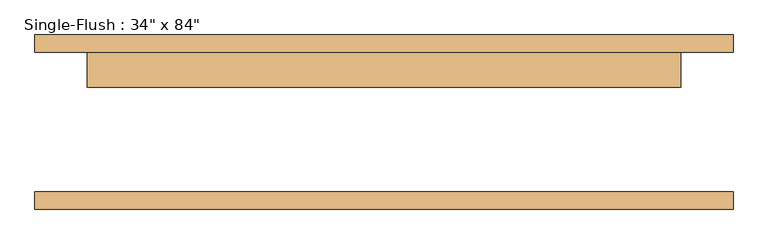
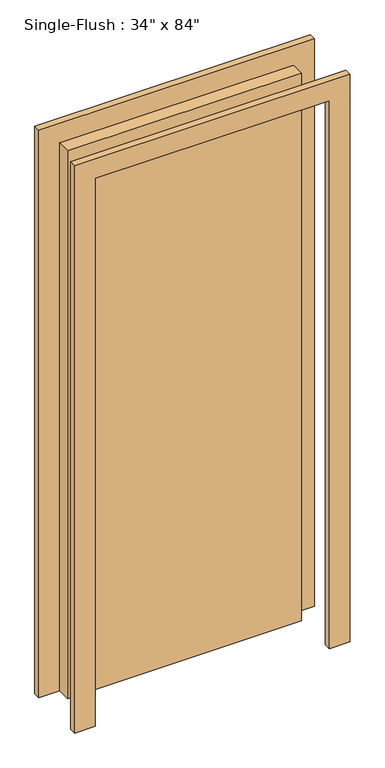
"""IFC4 building model written with IfcOpenShell, lengths in millimetres: door geometry."""

from ifc_helpers import new_model, si_unit, frame, origin, origin_with_axes, place, context, project, spatial, polyline, outline, extrude, source, transform, mapped, element, save


def door_f75d31f8(model_context):
    return source(origin(), model_context, "Body", "SweptSolid", [
        extrude(outline(polyline([(2209.8, -508.0), (0.0, -508.0), (0.0, -431.8), (2133.6, -431.8), (2133.6, 431.8), (0.0, 431.8), (0.0, 508.0), (2209.8, 508.0), (2209.8, -508.0)])), frame((0.0, 101.6, 0.0), z_axis=(0.0, 1.0, 0.0), x_axis=(0.0, 0.0, 1.0)), (0.0, 0.0, 1.0), 25.4),
        extrude(outline(polyline([(2209.8, 508.0), (2209.8, -508.0), (0.0, -508.0), (0.0, -431.8), (2133.6, -431.8), (2133.6, 431.8), (0.0, 431.8), (0.0, 508.0), (2209.8, 508.0)])), frame((0.0, -127.0, 0.0), z_axis=(0.0, 1.0, 0.0), x_axis=(0.0, 0.0, 1.0)), (0.0, 0.0, 1.0), 25.4),
        extrude(outline(polyline([(431.8, 50.8), (-431.8, 50.8), (-431.8, 101.6), (431.8, 101.6), (431.8, 50.8)])), origin_with_axes(), (0.0, 0.0, 1.0), 2133.6),
    ])


if __name__ == "__main__":
    model = new_model("IFC4")
    model_context = context("Model", 3, world=origin())
    ifc_project = project(units=[si_unit("LENGTHUNIT", "METRE", prefix="MILLI")], contexts=[model_context])
    site = spatial("IfcSite", under=ifc_project)
    building = spatial("IfcBuilding", under=site)
    placement = place(None, origin())
    door_shape = door_f75d31f8(model_context)
    element("IfcDoor", 1, ObjectType="Single-Flush : 34\" x 84\"", at=placement, inside=building, context=model_context, shape_type="MappedRepresentation", body=[
        mapped(door_shape, transform((0.0, 0.0, 0.0), x_axis=(1.0, 0.0, 0.0), y_axis=(0.0, 1.0, 0.0), z_axis=(0.0, 0.0, 1.0))),
    ])
    save(model, "model.ifc")

# Revit data of these elements
# Type "Single-Flush : 34\" x 84\""
#   Type Mark = "2"
#   Construction Type Id = "MDOOR"
#   Assembly Code = "C1020"
#   Analytic Construction = "Metal"
#   Thickness = 0' - 2"
#   Heat Transfer Coefficient (U) = 0.651978 BTU/(h·ft²·°F)
#   Height = 7' - 0"
#   Trim Projection Ext = 0' - 1"
#   Trim Projection Int = 0' - 1"
#   Trim Width = 0' - 3"
#   Width = 2' - 10"
#   Define Thermal Properties by = 1
#   Define Thermal Properties by = 1
#   Door Material = Door - Panel
#   Frame Material = Door - Frame
#   Visual Light Transmittance = 0
#   Solar Heat Gain Coefficient = 0
#   Function = (empty or 0)
#   Wall Closure = (empty or 0)
# Element 1 (IfcDoor, "Single-Flush : 34\" x 84\"")
#   Materials on its faces: "Door - Frame", "Door - Panel"
# Materials
#   "Door - Panel": class "Wood", colour RGB 210 159 95, transparency 0, Cost = 0
#   "Door - Frame": colour RGB 118 70 51, transparency 0, Cost = 0
